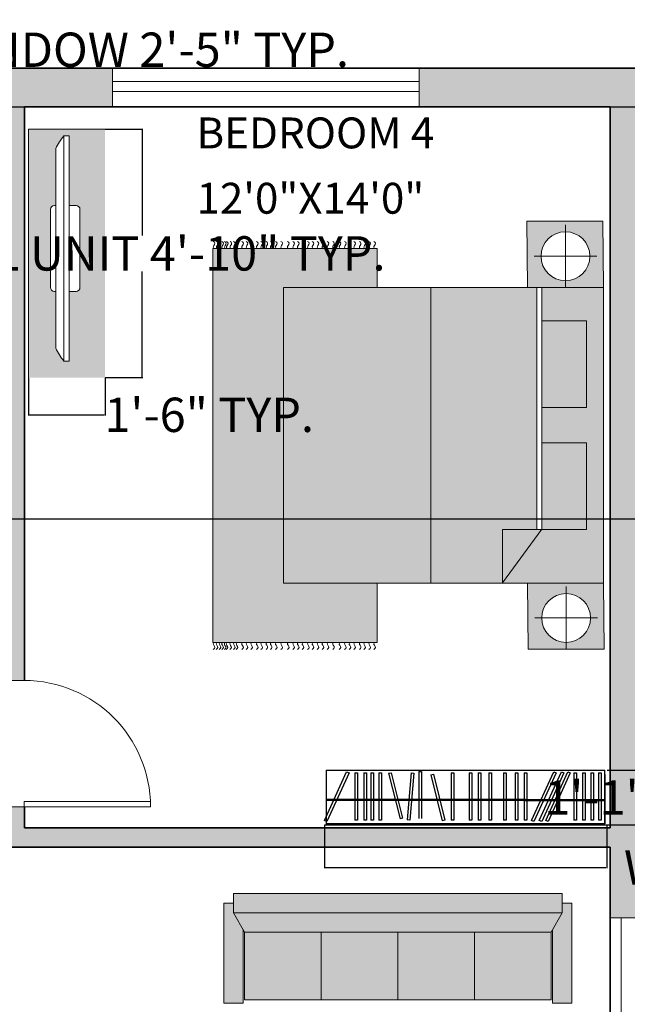
# Model space of a CAD drawing. Units: inches. Extents: x 853 to 1550, y 485 to 1596.
# Tile 16 of 18: x 1267 to 1409, y 1208 to 1437. Entities that reach past the tile are written whole.
import ezdxf

# ---------------------------------------------------------------- set-up
doc = ezdxf.new("R2010")
doc.units = ezdxf.units.IN
doc.header["$MEASUREMENT"] = 0
for name, color, linetype, lineweight in [('A-ANNO-DIMS', 2, 'Continuous', 18), ('A-AREA-IDEN', 250, 'Continuous', 18), ('A-DOOR', 4, 'Continuous', 18), ('A-WALL-PATT', 250, 'Continuous', 13), ('closet', 32, 'Continuous', 25), ('furniture', 250, 'Continuous', 18), ('walls', 250, 'Continuous', 35), ('windows', 4, 'Continuous', 18)]:
    doc.layers.add(name, color=color, linetype=linetype, lineweight=lineweight)
doc.layers.add('A-FURN-PATT', color=254, linetype='Continuous', lineweight=13, true_color=0xfeeab9)
doc.styles.get("Standard").update_dxf_attribs({"font": 'arial.ttf'})
doc.dimstyles.get("Standard").update_dxf_attribs({"dimtxt": 8, "dimasz": 0.18, "dimexe": 0.18, "dimexo": 0.0625, "dimgap": 0.09, "dimtad": 0, "dimtih": 1, "dimtoh": 1, "dimzin": 0, "dimdsep": 46, "dimlunit": 3, "dimtxsty": 'Standard', "dimcen": 0.09, "dimadec": 0, "dimazin": 0, "dimtfac": 1, "dimtofl": 0, "dimtmove": 0, "dimatfit": 3, "dimfxl": 1, "dimtolj": 1, "dimtzin": 0, "dimarcsym": 0})

# ---------------------------------------------------------------- blocks, each defined once
blk = doc.blocks.new('CARPET')
at = {"layer": 'furniture'}
for p, q in [((-51.53, -98.11), (-51.53, -55.12)), ((-51.53, -55.12), (-41.27, -55.12)), ((36, -55.12), (51.55, -55.12)), ((51.55, -55.12), (51.55, -98.11)), ((51.55, -98.11), (-51.53, -98.11))]:
    blk.add_line(p, q, dxfattribs=at)
for points, knots in [([(-53.37, -55.99), (-53.22, -55.8), (-52.9, -55.41), (-52.34, -55.8), (-51.89, -56.08), (-51.65, -55.91), (-51.53, -55.83)], [0, 0, 0, 0, 0.653278, 1.290138, 1.740457, 2.114451, 2.114451, 2.114451, 2.114451]), ([(53.37, -55.99), (53.22, -55.8), (52.9, -55.41), (52.34, -55.8), (51.89, -56.08), (51.65, -55.91), (51.53, -55.83)], [0, 0, 0, 0, 0.653278, 1.290138, 1.740457, 2.114451, 2.114451, 2.114451, 2.114451]), ([(-53.37, -57.26), (-53.22, -57.07), (-52.9, -56.67), (-52.34, -57.07), (-51.89, -57.35), (-51.65, -57.17), (-51.53, -57.1)], [0, 0, 0, 0, 0.653278, 1.290138, 1.740457, 2.114451, 2.114451, 2.114451, 2.114451]), ([(-53.37, -58.59), (-53.22, -58.4), (-52.9, -58.01), (-52.34, -58.4), (-51.89, -58.68), (-51.65, -58.5), (-51.53, -58.43)], [0, 0, 0, 0, 0.653278, 1.290138, 1.740457, 2.114451, 2.114451, 2.114451, 2.114451]), ([(53.37, -57.26), (53.22, -57.07), (52.9, -56.67), (52.34, -57.07), (51.89, -57.35), (51.65, -57.17), (51.53, -57.1)], [0, 0, 0, 0, 0.653278, 1.290138, 1.740457, 2.114451, 2.114451, 2.114451, 2.114451]), ([(53.37, -58.59), (53.22, -58.4), (52.9, -58.01), (52.34, -58.4), (51.89, -58.68), (51.65, -58.5), (51.53, -58.43)], [0, 0, 0, 0, 0.653278, 1.290138, 1.740457, 2.114451, 2.114451, 2.114451, 2.114451]), ([(-53.37, -59.78), (-53.22, -59.58), (-52.9, -59.19), (-52.34, -59.58), (-51.89, -59.86), (-51.65, -59.69), (-51.53, -59.61)], [0, 0, 0, 0, 0.653278, 1.290138, 1.740457, 2.114451, 2.114451, 2.114451, 2.114451]), ([(-53.37, -61.22), (-53.22, -61.02), (-52.9, -60.63), (-52.34, -61.02), (-51.89, -61.3), (-51.65, -61.13), (-51.53, -61.05)], [0, 0, 0, 0, 0.653278, 1.290138, 1.740457, 2.114451, 2.114451, 2.114451, 2.114451]), ([(53.37, -59.78), (53.22, -59.58), (52.9, -59.19), (52.34, -59.58), (51.89, -59.86), (51.65, -59.69), (51.53, -59.61)], [0, 0, 0, 0, 0.653278, 1.290138, 1.740457, 2.114451, 2.114451, 2.114451, 2.114451]), ([(53.37, -61.22), (53.22, -61.02), (52.9, -60.63), (52.34, -61.02), (51.89, -61.3), (51.65, -61.13), (51.53, -61.05)], [0, 0, 0, 0, 0.653278, 1.290138, 1.740457, 2.114451, 2.114451, 2.114451, 2.114451]), ([(-53.37, -62.44), (-53.22, -62.25), (-52.9, -61.86), (-52.34, -62.25), (-51.89, -62.53), (-51.65, -62.36), (-51.53, -62.28)], [0, 0, 0, 0, 0.653278, 1.290138, 1.740457, 2.114451, 2.114451, 2.114451, 2.114451]), ([(-53.37, -63.63), (-53.22, -63.43), (-52.9, -63.04), (-52.34, -63.43), (-51.89, -63.72), (-51.65, -63.54), (-51.53, -63.46)], [0, 0, 0, 0, 0.653278, 1.290138, 1.740457, 2.114451, 2.114451, 2.114451, 2.114451]), ([(53.37, -62.44), (53.22, -62.25), (52.9, -61.86), (52.34, -62.25), (51.89, -62.53), (51.65, -62.36), (51.53, -62.28)], [0, 0, 0, 0, 0.653278, 1.290138, 1.740457, 2.114451, 2.114451, 2.114451, 2.114451]), ([(53.37, -63.63), (53.22, -63.43), (52.9, -63.04), (52.34, -63.43), (51.89, -63.72), (51.65, -63.54), (51.53, -63.46)], [0, 0, 0, 0, 0.653278, 1.290138, 1.740457, 2.114451, 2.114451, 2.114451, 2.114451]), ([(-53.37, -65.07), (-53.22, -64.87), (-52.9, -64.48), (-52.34, -64.87), (-51.89, -65.15), (-51.65, -64.98), (-51.53, -64.9)], [0, 0, 0, 0, 0.653278, 1.290138, 1.740457, 2.114451, 2.114451, 2.114451, 2.114451]), ([(-53.37, -66.76), (-53.22, -66.56), (-52.9, -66.17), (-52.34, -66.56), (-51.89, -66.84), (-51.65, -66.67), (-51.53, -66.59)], [0, 0, 0, 0, 0.653278, 1.290138, 1.740457, 2.114451, 2.114451, 2.114451, 2.114451]), ([(53.37, -65.07), (53.22, -64.87), (52.9, -64.48), (52.34, -64.87), (51.89, -65.15), (51.65, -64.98), (51.53, -64.9)], [0, 0, 0, 0, 0.653278, 1.290138, 1.740457, 2.114451, 2.114451, 2.114451, 2.114451]), ([(53.37, -66.76), (53.22, -66.56), (52.9, -66.17), (52.34, -66.56), (51.89, -66.84), (51.65, -66.67), (51.53, -66.59)], [0, 0, 0, 0, 0.653278, 1.290138, 1.740457, 2.114451, 2.114451, 2.114451, 2.114451]), ([(-53.37, -68.2), (-53.22, -68), (-52.9, -67.61), (-52.34, -68), (-51.89, -68.28), (-51.65, -68.11), (-51.53, -68.03)], [0, 0, 0, 0, 0.653278, 1.290138, 1.740457, 2.114451, 2.114451, 2.114451, 2.114451]), ([(-53.37, -69.53), (-53.22, -69.33), (-52.9, -68.94), (-52.34, -69.33), (-51.89, -69.61), (-51.65, -69.44), (-51.53, -69.36)], [0, 0, 0, 0, 0.653278, 1.290138, 1.740457, 2.114451, 2.114451, 2.114451, 2.114451]), ([(53.37, -68.2), (53.22, -68), (52.9, -67.61), (52.34, -68), (51.89, -68.28), (51.65, -68.11), (51.53, -68.03)], [0, 0, 0, 0, 0.653278, 1.290138, 1.740457, 2.114451, 2.114451, 2.114451, 2.114451]), ([(53.37, -69.53), (53.22, -69.33), (52.9, -68.94), (52.34, -69.33), (51.89, -69.61), (51.65, -69.44), (51.53, -69.36)], [0, 0, 0, 0, 0.653278, 1.290138, 1.740457, 2.114451, 2.114451, 2.114451, 2.114451]), ([(-53.37, -70.79), (-53.22, -70.6), (-52.9, -70.21), (-52.34, -70.6), (-51.89, -70.88), (-51.65, -70.7), (-51.53, -70.63)], [0, 0, 0, 0, 0.653278, 1.290138, 1.740457, 2.114451, 2.114451, 2.114451, 2.114451]), ([(-53.37, -72.12), (-53.22, -71.93), (-52.9, -71.54), (-52.34, -71.93), (-51.89, -72.21), (-51.65, -72.04), (-51.53, -71.96)], [0, 0, 0, 0, 0.653278, 1.290138, 1.740457, 2.114451, 2.114451, 2.114451, 2.114451]), ([(53.37, -70.79), (53.22, -70.6), (52.9, -70.21), (52.34, -70.6), (51.89, -70.88), (51.65, -70.7), (51.53, -70.63)], [0, 0, 0, 0, 0.653278, 1.290138, 1.740457, 2.114451, 2.114451, 2.114451, 2.114451]), ([(53.37, -72.12), (53.22, -71.93), (52.9, -71.54), (52.34, -71.93), (51.89, -72.21), (51.65, -72.04), (51.53, -71.96)], [0, 0, 0, 0, 0.653278, 1.290138, 1.740457, 2.114451, 2.114451, 2.114451, 2.114451]), ([(-53.37, -73.31), (-53.22, -73.11), (-52.9, -72.72), (-52.34, -73.11), (-51.89, -73.4), (-51.65, -73.22), (-51.53, -73.14)], [0, 0, 0, 0, 0.653278, 1.290138, 1.740457, 2.114451, 2.114451, 2.114451, 2.114451]), ([(-53.37, -74.75), (-53.22, -74.55), (-52.9, -74.16), (-52.34, -74.55), (-51.89, -74.83), (-51.65, -74.66), (-51.53, -74.58)], [0, 0, 0, 0, 0.653278, 1.290138, 1.740457, 2.114451, 2.114451, 2.114451, 2.114451]), ([(53.37, -73.31), (53.22, -73.11), (52.9, -72.72), (52.34, -73.11), (51.89, -73.4), (51.65, -73.22), (51.53, -73.14)], [0, 0, 0, 0, 0.653278, 1.290138, 1.740457, 2.114451, 2.114451, 2.114451, 2.114451]), ([(53.37, -74.75), (53.22, -74.55), (52.9, -74.16), (52.34, -74.55), (51.89, -74.83), (51.65, -74.66), (51.53, -74.58)], [0, 0, 0, 0, 0.653278, 1.290138, 1.740457, 2.114451, 2.114451, 2.114451, 2.114451]), ([(-53.37, -75.98), (-53.22, -75.78), (-52.9, -75.39), (-52.34, -75.78), (-51.89, -76.06), (-51.65, -75.89), (-51.53, -75.81)], [0, 0, 0, 0, 0.653278, 1.290138, 1.740457, 2.114451, 2.114451, 2.114451, 2.114451]), ([(-53.37, -77.16), (-53.22, -76.96), (-52.9, -76.57), (-52.34, -76.96), (-51.89, -77.25), (-51.65, -77.07), (-51.53, -76.99)], [0, 0, 0, 0, 0.653278, 1.290138, 1.740457, 2.114451, 2.114451, 2.114451, 2.114451]), ([(53.37, -75.98), (53.22, -75.78), (52.9, -75.39), (52.34, -75.78), (51.89, -76.06), (51.65, -75.89), (51.53, -75.81)], [0, 0, 0, 0, 0.653278, 1.290138, 1.740457, 2.114451, 2.114451, 2.114451, 2.114451]), ([(53.37, -77.16), (53.22, -76.96), (52.9, -76.57), (52.34, -76.96), (51.89, -77.25), (51.65, -77.07), (51.53, -76.99)], [0, 0, 0, 0, 0.653278, 1.290138, 1.740457, 2.114451, 2.114451, 2.114451, 2.114451]), ([(-53.37, -78.6), (-53.22, -78.4), (-52.9, -78.01), (-52.34, -78.4), (-51.89, -78.68), (-51.65, -78.51), (-51.53, -78.43)], [0, 0, 0, 0, 0.653278, 1.290138, 1.740457, 2.114451, 2.114451, 2.114451, 2.114451]), ([(53.37, -78.6), (53.22, -78.4), (52.9, -78.01), (52.34, -78.4), (51.89, -78.68), (51.65, -78.51), (51.53, -78.43)], [0, 0, 0, 0, 0.653278, 1.290138, 1.740457, 2.114451, 2.114451, 2.114451, 2.114451]), ([(-53.37, -80.29), (-53.22, -80.09), (-52.9, -79.7), (-52.34, -80.09), (-51.89, -80.37), (-51.65, -80.2), (-51.53, -80.12)], [0, 0, 0, 0, 0.653278, 1.290138, 1.740457, 2.114451, 2.114451, 2.114451, 2.114451]), ([(-53.37, -81.73), (-53.22, -81.53), (-52.9, -81.14), (-52.34, -81.53), (-51.89, -81.81), (-51.65, -81.64), (-51.53, -81.56)], [0, 0, 0, 0, 0.653278, 1.290138, 1.740457, 2.114451, 2.114451, 2.114451, 2.114451]), ([(53.37, -80.29), (53.22, -80.09), (52.9, -79.7), (52.34, -80.09), (51.89, -80.37), (51.65, -80.2), (51.53, -80.12)], [0, 0, 0, 0, 0.653278, 1.290138, 1.740457, 2.114451, 2.114451, 2.114451, 2.114451]), ([(53.37, -81.73), (53.22, -81.53), (52.9, -81.14), (52.34, -81.53), (51.89, -81.81), (51.65, -81.64), (51.53, -81.56)], [0, 0, 0, 0, 0.653278, 1.290138, 1.740457, 2.114451, 2.114451, 2.114451, 2.114451]), ([(-53.37, -83.06), (-53.22, -82.86), (-52.9, -82.47), (-52.34, -82.86), (-51.89, -83.14), (-51.65, -82.97), (-51.53, -82.89)], [0, 0, 0, 0, 0.653278, 1.290138, 1.740457, 2.114451, 2.114451, 2.114451, 2.114451]), ([(-53.37, -84.18), (-53.22, -83.99), (-52.9, -83.6), (-52.34, -83.99), (-51.89, -84.27), (-51.65, -84.09), (-51.53, -84.02)], [0, 0, 0, 0, 0.653278, 1.290138, 1.740457, 2.114451, 2.114451, 2.114451, 2.114451]), ([(53.37, -83.06), (53.22, -82.86), (52.9, -82.47), (52.34, -82.86), (51.89, -83.14), (51.65, -82.97), (51.53, -82.89)], [0, 0, 0, 0, 0.653278, 1.290138, 1.740457, 2.114451, 2.114451, 2.114451, 2.114451]), ([(53.37, -84.18), (53.22, -83.99), (52.9, -83.6), (52.34, -83.99), (51.89, -84.27), (51.65, -84.09), (51.53, -84.02)], [0, 0, 0, 0, 0.653278, 1.290138, 1.740457, 2.114451, 2.114451, 2.114451, 2.114451]), ([(-53.37, -85.51), (-53.22, -85.32), (-52.9, -84.93), (-52.34, -85.32), (-51.89, -85.6), (-51.65, -85.42), (-51.53, -85.35)], [0, 0, 0, 0, 0.653278, 1.290138, 1.740457, 2.114451, 2.114451, 2.114451, 2.114451]), ([(-53.37, -86.7), (-53.22, -86.5), (-52.9, -86.11), (-52.34, -86.5), (-51.89, -86.78), (-51.65, -86.61), (-51.53, -86.53)], [0, 0, 0, 0, 0.653278, 1.290138, 1.740457, 2.114451, 2.114451, 2.114451, 2.114451]), ([(53.37, -85.51), (53.22, -85.32), (52.9, -84.93), (52.34, -85.32), (51.89, -85.6), (51.65, -85.42), (51.53, -85.35)], [0, 0, 0, 0, 0.653278, 1.290138, 1.740457, 2.114451, 2.114451, 2.114451, 2.114451]), ([(53.37, -86.7), (53.22, -86.5), (52.9, -86.11), (52.34, -86.5), (51.89, -86.78), (51.65, -86.61), (51.53, -86.53)], [0, 0, 0, 0, 0.653278, 1.290138, 1.740457, 2.114451, 2.114451, 2.114451, 2.114451]), ([(-53.37, -88.14), (-53.22, -87.94), (-52.9, -87.55), (-52.34, -87.94), (-51.89, -88.22), (-51.65, -88.05), (-51.53, -87.97)], [0, 0, 0, 0, 0.653278, 1.290138, 1.740457, 2.114451, 2.114451, 2.114451, 2.114451]), ([(-53.37, -89.36), (-53.22, -89.17), (-52.9, -88.78), (-52.34, -89.17), (-51.89, -89.45), (-51.65, -89.28), (-51.53, -89.2)], [0, 0, 0, 0, 0.653278, 1.290138, 1.740457, 2.114451, 2.114451, 2.114451, 2.114451]), ([(-53.37, -90.55), (-53.22, -90.35), (-52.9, -89.96), (-52.34, -90.35), (-51.89, -90.64), (-51.65, -90.46), (-51.53, -90.38)], [0, 0, 0, 0, 0.653278, 1.290138, 1.740457, 2.114451, 2.114451, 2.114451, 2.114451]), ([(53.37, -88.14), (53.22, -87.94), (52.9, -87.55), (52.34, -87.94), (51.89, -88.22), (51.65, -88.05), (51.53, -87.97)], [0, 0, 0, 0, 0.653278, 1.290138, 1.740457, 2.114451, 2.114451, 2.114451, 2.114451]), ([(53.37, -89.36), (53.22, -89.17), (52.9, -88.78), (52.34, -89.17), (51.89, -89.45), (51.65, -89.28), (51.53, -89.2)], [0, 0, 0, 0, 0.653278, 1.290138, 1.740457, 2.114451, 2.114451, 2.114451, 2.114451]), ([(53.37, -90.55), (53.22, -90.35), (52.9, -89.96), (52.34, -90.35), (51.9, -90.63), (51.66, -90.47), (51.55, -90.4)], [0, 0, 0, 0, 0.653278, 1.290138, 1.740457, 2.0926, 2.0926, 2.0926, 2.0926]), ([(-53.37, -91.99), (-53.22, -91.79), (-52.9, -91.4), (-52.34, -91.79), (-51.89, -92.07), (-51.65, -91.9), (-51.53, -91.82)], [0, 0, 0, 0, 0.653278, 1.290138, 1.740457, 2.114451, 2.114451, 2.114451, 2.114451]), ([(-53.37, -92.69), (-53.22, -92.48), (-52.9, -92.08), (-52.35, -92.49), (-51.89, -92.77), (-51.65, -92.6), (-51.53, -92.52)], [0, 0, 0, 0, 0.663904, 1.307406, 1.757725, 2.131719, 2.131719, 2.131719, 2.131719]), ([(53.37, -91.99), (53.22, -91.79), (52.9, -91.4), (52.34, -91.79), (51.9, -92.07), (51.66, -91.91), (51.55, -91.83)], [0, 0, 0, 0, 0.653278, 1.290138, 1.740457, 2.0926, 2.0926, 2.0926, 2.0926]), ([(53.37, -92.69), (53.22, -92.49), (52.9, -92.09), (52.34, -92.49), (51.9, -92.77), (51.66, -92.61), (51.55, -92.53)], [0, 0, 0, 0, 0.656792, 1.295826, 1.746145, 2.098292, 2.098292, 2.098292, 2.098292]), ([(-53.37, -93.61), (-53.22, -93.42), (-52.9, -93.03), (-52.34, -93.42), (-51.89, -93.7), (-51.65, -93.52), (-51.53, -93.45)], [0, 0, 0, 0, 0.653278, 1.290138, 1.740457, 2.114451, 2.114451, 2.114451, 2.114451]), ([(-53.37, -94.55), (-53.22, -94.35), (-52.9, -93.96), (-52.34, -94.35), (-51.89, -94.63), (-51.65, -94.46), (-51.53, -94.38)], [0, 0, 0, 0, 0.653278, 1.290138, 1.740457, 2.114451, 2.114451, 2.114451, 2.114451]), ([(-53.37, -95.05), (-53.22, -94.85), (-52.9, -94.46), (-52.34, -94.85), (-51.89, -95.14), (-51.65, -94.96), (-51.53, -94.88)], [0, 0, 0, 0, 0.653278, 1.290138, 1.740457, 2.114451, 2.114451, 2.114451, 2.114451]), ([(53.37, -93.66), (53.22, -93.46), (52.9, -93.07), (52.34, -93.46), (51.9, -93.74), (51.66, -93.58), (51.55, -93.5)], [0, 0, 0, 0, 0.653278, 1.290138, 1.740457, 2.0926, 2.0926, 2.0926, 2.0926]), ([(53.37, -94.59), (53.22, -94.4), (52.9, -94.01), (52.34, -94.4), (51.9, -94.68), (51.66, -94.51), (51.55, -94.44)], [0, 0, 0, 0, 0.653278, 1.290138, 1.740457, 2.0926, 2.0926, 2.0926, 2.0926]), ([(53.37, -95.1), (53.22, -94.9), (52.9, -94.51), (52.34, -94.9), (51.9, -95.18), (51.66, -95.02), (51.55, -94.94)], [0, 0, 0, 0, 0.653278, 1.290138, 1.740457, 2.0926, 2.0926, 2.0926, 2.0926]), ([(-53.37, -95.73), (-53.22, -95.54), (-52.9, -95.15), (-52.34, -95.54), (-51.89, -95.82), (-51.65, -95.65), (-51.53, -95.57)], [0, 0, 0, 0, 0.653278, 1.290138, 1.740457, 2.114451, 2.114451, 2.114451, 2.114451]), ([(-53.37, -96.38), (-53.22, -96.18), (-52.9, -95.79), (-52.34, -96.18), (-51.89, -96.47), (-51.65, -96.29), (-51.53, -96.21)], [0, 0, 0, 0, 0.653278, 1.290138, 1.740457, 2.114451, 2.114451, 2.114451, 2.114451]), ([(-53.37, -97.17), (-53.22, -96.98), (-52.9, -96.59), (-52.34, -96.98), (-51.89, -97.26), (-51.65, -97.08), (-51.53, -97.01)], [0, 0, 0, 0, 0.653278, 1.290138, 1.740457, 2.114451, 2.114451, 2.114451, 2.114451]), ([(-53.37, -97.99), (-53.22, -97.79), (-52.9, -97.4), (-52.34, -97.79), (-51.89, -98.08), (-51.65, -97.9), (-51.53, -97.82)], [0, 0, 0, 0, 0.653278, 1.290138, 1.740457, 2.114451, 2.114451, 2.114451, 2.114451]), ([(53.37, -95.78), (53.22, -95.58), (52.9, -95.19), (52.34, -95.58), (51.89, -95.86), (51.65, -95.69), (51.53, -95.61)], [0, 0, 0, 0, 0.653278, 1.290138, 1.740457, 2.114451, 2.114451, 2.114451, 2.114451]), ([(53.37, -96.43), (53.22, -96.23), (52.9, -95.84), (52.34, -96.23), (51.89, -96.51), (51.65, -96.34), (51.53, -96.26)], [0, 0, 0, 0, 0.653278, 1.290138, 1.740457, 2.114451, 2.114451, 2.114451, 2.114451]), ([(53.37, -97.22), (53.22, -97.02), (52.9, -96.63), (52.34, -97.02), (51.89, -97.3), (51.65, -97.13), (51.53, -97.05)], [0, 0, 0, 0, 0.653278, 1.290138, 1.740457, 2.114451, 2.114451, 2.114451, 2.114451]), ([(53.37, -97.99), (53.22, -97.79), (52.9, -97.4), (52.34, -97.79), (51.89, -98.08), (51.65, -97.9), (51.53, -97.82)], [0, 0, 0, 0, 0.653278, 1.290138, 1.740457, 2.114451, 2.114451, 2.114451, 2.114451])]:
    blk.add_open_spline(points, degree=3, knots=knots, dxfattribs=at)
blk = doc.blocks.new('A$C58D270C6')
at = {"layer": 'furniture'}
for p, q in [((9.09, 124.13), (9.09, 108.87)), ((1.46, 116.5), (16.73, 116.5)), ((42.08, 108), (42.08, 36)), ((14.97, 94.84), (24.62, 107.92)), ((24.62, 94.93), (24.62, 107.92)), ((14.97, 94.93), (24.62, 94.93)), ((14.97, 94.84), (14.97, 36)), ((16.22, 94.93), (16.22, 36)), ((9.25, 36), (9.25, 20.74)), ((1.62, 28.37), (16.88, 28.37))]:
    blk.add_line(p, q, dxfattribs=at)
for points in [[(18.5, 108), (18.34, 124.13), (-0.16, 124.13), (0, 108)], [(0, 108), (77.91, 108), (77.91, 36), (0, 36)], [(4.09, 94.93), (14.97, 94.93), (14.97, 73.83), (4.09, 73.83)], [(4.09, 65.23), (14.97, 65.23), (14.97, 44.13), (4.09, 44.13)], [(18.65, 19.87), (18.5, 36), (0, 36), (0.16, 19.87)]]:
    blk.add_lwpolyline(points, close=True, dxfattribs=at)
for centre in [(9.09, 116.5), (9.25, 28.37)]:
    blk.add_circle(centre, 5.95, dxfattribs=at)
at = {"layer": 'furniture', "xscale": 0.9312884925094044, "yscale": 0.9312884925094044, "zscale": 0.9312884925094044, "rotation": 90}
blk.add_blockref('CARPET', (3.79, 74.47), dxfattribs=at)
blk = doc.blocks.new('*U10')
for p, q in [((0, 0), (0, -6)), ((40, 0), (40, -6))]:
    blk.add_line(p, q)
blk.add_lwpolyline([(0, 0), (0, 40), (1.75, 40), (1.75, 0)], close=True)
blk.add_arc((0, 0), 40, 0, 90)
blk = doc.blocks.new('FABRIC SOFA 4S')
at = {"layer": 'furniture'}
for p, q in [((3, 54), (34, 54)), ((3, 51), (3, 54)), ((34, 48), (34, 54)), ((0, -51), (0, 51)), ((6, 51), (0, 51)), ((6, -51), (6, 51)), ((12, 47.63), (6, 51)), ((11.14, 48), (34, 48)), ((33, 23.81), (12, 23.81)), ((33, 0), (12, 0)), ((33, -23.81), (12, -23.81)), ((6, -51), (12, -47.63)), ((11.54, -48), (34, -48)), ((34, -48), (34, -54)), ((6, -51), (0, -51)), ((3, -54), (3, -51)), ((3, -54), (34, -54))]:
    blk.add_line(p, q, dxfattribs=at)
blk.add_lwpolyline([(12, -47.63), (12, 47.63), (33, 47.63), (33, -47.63)], close=True, dxfattribs=at)
blk = doc.blocks.new('WIN-71IN')
for p, q in [((0, 9), (0, 0)), ((71.43, 9), (0, 9)), ((0, 9), (0, 5.92)), ((71.43, 0), (71.43, 9)), ((0, 5.92), (71.43, 5.92)), ((71.43, 5.92), (71.43, 3.59)), ((71.43, 3.59), (0, 3.59)), ((0, 0), (71.43, 0))]:
    blk.add_line(p, q)
blk = doc.blocks.new('WIN-94IN')
for p, q in [((0, 94.25), (9, 94.25)), ((0, 0), (0, 94.25)), ((2.54, 94.25), (2.54, 0)), ((6.1, 0), (6.1, 94.25)), ((9, 94.25), (9, 0)), ((9, 0), (0, 0)), ((2.54, 0), (6.1, 0))]:
    blk.add_line(p, q)
blk = doc.blocks.new('closet')
at = {"layer": 'closet'}
for p, q in [((-0.71, -5.58), (5.59, 8.19)), ((-0.23, 7.39), (-0.23, -6.57)), ((6.27, 7.88), (-0.04, -5.89)), ((5.59, 8.19), (6.27, 7.88)), ((7.92, 7.84), (8.68, 7.84)), ((7.92, 7.84), (7.92, -5.51)), ((8.68, 7.84), (8.68, -5.51)), ((10.44, 7.84), (11.2, 7.84)), ((10.44, 7.84), (10.44, -5.51)), ((11.2, 7.84), (11.2, -5.51)), ((12.45, 7.84), (13.21, 7.84)), ((12.45, 7.84), (12.45, -5.51)), ((13.21, 7.84), (13.21, -5.51)), ((14.71, 7.84), (15.47, 7.84)), ((14.71, 7.84), (14.71, -5.51)), ((15.47, 7.84), (15.47, -5.51)), ((17.44, 7.75), (18.17, 7.93)), ((17.44, 7.75), (20.73, -5.2)), ((18.17, 7.93), (21.46, -5.01)), ((23.92, 7.84), (22.75, -5.46)), ((24.67, 7.78), (23.51, -5.53)), ((23.92, 7.84), (24.67, 7.78)), ((26.09, 8.25), (26.09, -5.1)), ((26.84, 8.25), (26.84, -5.1)), ((29.49, 7.29), (32.64, -5.69)), ((30.22, 7.46), (33.37, -5.51)), ((35.23, 7.84), (35.23, -5.51)), ((35.99, 7.84), (35.99, -5.51)), ((40.33, 7.84), (40.33, -5.51)), ((41.08, 7.84), (41.08, -5.51)), ((42.85, 7.84), (42.85, -5.51)), ((43.61, 7.84), (43.61, -5.51)), ((45.9, 7.84), (45.9, -5.51)), ((46.65, 7.84), (46.65, -5.51)), ((50.07, 7.84), (50.07, -5.51)), ((50.82, 7.84), (50.82, -5.51)), ((53.32, 7.84), (53.32, -5.51)), ((54.08, 7.84), (54.08, -5.51)), ((55.9, 7.84), (55.9, -5.51)), ((56.65, 7.84), (56.65, -5.51)), ((57.99, -5.58), (64.3, 8.19)), ((64.97, 7.88), (58.67, -5.89)), ((60.19, -5.58), (66.49, 8.19)), ((67.17, 7.88), (60.87, -5.89)), ((62, -5.58), (68.3, 8.19)), ((68.98, 7.88), (62.67, -5.89)), ((69.96, 7.84), (69.96, -5.51)), ((70.72, 7.84), (70.72, -5.51)), ((72.43, 7.84), (72.43, -5.51)), ((73.19, 7.84), (73.19, -5.51)), ((74.82, 7.84), (74.82, -5.51)), ((75.57, 7.84), (75.57, -5.51)), ((76.94, 7.84), (76.94, -5.51)), ((77.69, 7.84), (77.69, -5.51)), ((56.23, 0.33), (0, 0.33)), ((56.2, 0), (0, 0)), ((56.2, 0), (78.76, 0)), ((56.23, 0.33), (78.76, 0.33)), ((-0.04, -5.89), (-0.71, -5.58)), ((21.46, -5.01), (20.73, -5.2)), ((23.51, -5.53), (22.75, -5.46)), ((33.37, -5.51), (32.64, -5.69)), ((35.99, -5.51), (35.23, -5.51)), ((41.08, -5.51), (40.33, -5.51)), ((43.61, -5.51), (42.85, -5.51)), ((46.65, -5.51), (45.9, -5.51)), ((50.82, -5.51), (50.07, -5.51)), ((54.08, -5.51), (53.32, -5.51)), ((56.65, -5.51), (55.9, -5.51)), ((58.67, -5.89), (57.99, -5.58)), ((60.87, -5.89), (60.19, -5.58)), ((62.67, -5.89), (62, -5.58)), ((70.72, -5.51), (69.96, -5.51)), ((73.19, -5.51), (72.43, -5.51)), ((75.57, -5.51), (74.82, -5.51)), ((77.69, -5.51), (76.94, -5.51))]:
    blk.add_line(p, q, dxfattribs=at)
blk = doc.blocks.new('rotated closet')
at = {"layer": 'closet'}
for p, q in [((26.32, 0.86), (27.07, 0.86)), ((29.72, -0.11), (30.45, 0.07)), ((35.46, 0.45), (36.22, 0.45)), ((40.56, 0.45), (41.31, 0.45)), ((43.08, 0.45), (43.84, 0.45)), ((46.13, 0.45), (46.88, 0.45)), ((50.3, 0.45), (51.05, 0.45)), ((53.56, 0.45), (54.31, 0.45)), ((56.13, 0.45), (56.88, 0.45)), ((64.53, 0.8), (65.2, 0.49)), ((66.72, 0.8), (67.4, 0.49)), ((68.53, 0.8), (69.21, 0.49)), ((70.19, 0.45), (70.95, 0.45)), ((72.66, 0.45), (73.42, 0.45)), ((75.05, 0.45), (75.81, 0.45)), ((77.17, 0.45), (77.92, 0.45)), ((78.99, 0), (78.99, -13.96)), ((8.91, -12.91), (8.15, -12.91)), ((11.43, -12.91), (10.67, -12.91)), ((13.44, -12.91), (12.68, -12.91)), ((15.7, -12.91), (14.94, -12.91)), ((-0.46, -14.27), (79.54, -14.27)), ((0, -13.96), (78.99, -13.96))]:
    blk.add_line(p, q, dxfattribs=at)
blk.add_blockref('closet', (0.23, -7.39), dxfattribs=at)
blk = doc.blocks.new('WARDROBE-FRAMED')
for p, q in [((0.4, 12.8), (65.33, 12.8)), ((0.4, 12.8), (0.4, 0.26)), ((65.33, 0.26), (65.33, 12.8)), ((0.02, 0), (65.79, 0)), ((65.33, 0.26), (0.4, 0.26)), ((0.4, 0.26), (0.4, 0))]:
    blk.add_line(p, q)
at = {"xscale": 0.8221057635095903, "yscale": 0.8221057635095903, "zscale": 0.8221057635095903, "rotation": 359.9999999992008}
blk.add_blockref('rotated closet', (0.4, 11.74), dxfattribs=at)
blk = doc.blocks.new('PLASMA-LARGE')
at = {"layer": 'furniture'}
for p, q in [((-7.26, 0), (7.26, 0)), ((-18.61, -1), (18.61, -1)), ((-8, -1), (-8, -0.74)), ((8, -1), (8, -0.74)), ((-21, -2.5), (21, -2.5)), ((-21, -2.5), (-21, -3.5)), ((-21, -3.5), (21, -3.5)), ((-8, -3.5), (-8, -4.76)), ((8, -3.5), (8, -4.76)), ((21, -2.5), (21, -3.5)), ((-7.26, -5.5), (7.26, -5.5))]:
    blk.add_line(p, q, dxfattribs=at)
for centre, radius, start, end in [((-7.26, -0.74), 0.744, 90, 180), ((7.26, -0.74), 0.744, 0, 90), ((-13.97, -11.05), 11.07, 114.7602, 129.4175), ((13.97, -11.05), 11.07, 50.5825, 65.2398), ((-7.26, -4.76), 0.744, 180, 270), ((7.26, -4.76), 0.744, 270, 0)]:
    blk.add_arc(centre, radius, start, end, dxfattribs=at)
blk = doc.blocks.new('TV-CONSOLE-WALL')
for p, q in [((17.81, 57.83), (0, 57.83)), ((0, 57.83), (0, 0))]:
    blk.add_line(p, q)
at = {"xscale": -1.249763490704796, "yscale": 1.249763490704796, "zscale": 1.249763490704796, "rotation": 90}
blk.add_blockref('PLASMA-LARGE', (5.11, 30.08), dxfattribs=at)
blk = doc.blocks.new('*D43')
at = {"layer": 'A-ANNO-DIMS', "color": 0, "lineweight": -2, "transparency": 16777216}
for p, q in [((1338.32, 1249.77), (1338.32, 1239.78)), ((1404.11, 1249.77), (1404.11, 1239.78)), ((1338.5, 1239.96), (1403.93, 1239.96)), ((1404.11, 1239.96), (1404.29, 1239.96))]:
    blk.add_line(p, q, dxfattribs=at)
at = {"layer": 'A-ANNO-DIMS', "color": 0, "transparency": 16777216}
for points in [[(1338.5, 1239.99), (1338.5, 1239.93), (1338.32, 1239.96)], [(1403.93, 1239.99), (1403.93, 1239.93), (1404.11, 1239.96)]]:
    blk.add_solid(points, dxfattribs=at)
at = {"layer": 'Defpoints', "color": 0, "transparency": 16777216}
for p in [(1338.32, 1249.83), (1404.11, 1249.83), (1404.11, 1239.96)]:
    blk.add_point(p, dxfattribs=at)
at = {"layer": 'A-ANNO-DIMS', "color": 0, "transparency": 16777216, "insert": (1463.39, 1239.96), "char_height": 8, "attachment_point": 5}
blk.add_mtext('\\A1;WARDROBE 5\'-6" TYP.', dxfattribs=at)
blk = doc.blocks.new('*D44')
at = {"layer": 'A-ANNO-DIMS', "color": 0, "lineweight": -2, "transparency": 16777216}
for p, q in [((1404.17, 1262.63), (1414.16, 1262.63)), ((1413.98, 1262.45), (1413.98, 1260.34)), ((1413.98, 1250.01), (1413.98, 1252.12)), ((1404.17, 1249.83), (1414.16, 1249.83))]:
    blk.add_line(p, q, dxfattribs=at)
at = {"layer": 'A-ANNO-DIMS', "color": 0, "transparency": 16777216}
for points in [[(1413.95, 1262.45), (1414.01, 1262.45), (1413.98, 1262.63)], [(1413.95, 1250.01), (1414.01, 1250.01), (1413.98, 1249.83)]]:
    blk.add_solid(points, dxfattribs=at)
at = {"layer": 'Defpoints', "color": 0, "transparency": 16777216}
for p in [(1404.11, 1262.63), (1413.98, 1262.63), (1404.11, 1249.83)]:
    blk.add_point(p, dxfattribs=at)
at = {"layer": 'A-ANNO-DIMS', "color": 0, "transparency": 16777216, "insert": (1413.98, 1256.23), "char_height": 8, "attachment_point": 5}
blk.add_mtext('\\A1;1\'-1" TYP.', dxfattribs=at)
blk = doc.blocks.new('*D51')
at = {"layer": 'A-ANNO-DIMS', "color": 0, "lineweight": -2, "transparency": 16777216}
for p, q in [((1215.84, 1426.19), (1215.84, 1430.62)), ((1216.02, 1430.44), (1244.42, 1430.44)), ((1244.6, 1426.19), (1244.6, 1430.62)), ((1244.6, 1430.44), (1244.78, 1430.44))]:
    blk.add_line(p, q, dxfattribs=at)
at = {"layer": 'A-ANNO-DIMS', "color": 0, "transparency": 16777216}
for points in [[(1216.02, 1430.47), (1216.02, 1430.41), (1215.84, 1430.44)], [(1244.42, 1430.47), (1244.42, 1430.41), (1244.6, 1430.44)]]:
    blk.add_solid(points, dxfattribs=at)
at = {"layer": 'Defpoints', "color": 0, "transparency": 16777216}
for p in [(1244.6, 1430.44), (1215.84, 1426.13), (1244.6, 1426.13)]:
    blk.add_point(p, dxfattribs=at)
at = {"layer": 'A-ANNO-DIMS', "color": 0, "transparency": 16777216, "insert": (1295.48, 1430.44), "char_height": 8, "attachment_point": 5}
blk.add_mtext('\\A1;WINDOW 2\'-5" TYP.', dxfattribs=at)
blk = doc.blocks.new('*D57')
at = {"layer": 'A-ANNO-DIMS', "color": 0, "lineweight": -2, "transparency": 16777216}
for p, q in [((1287.27, 1411.9), (1296.06, 1411.9)), ((1295.88, 1411.72), (1295.88, 1387.16)), ((1295.88, 1354.25), (1295.88, 1378.81)), ((1287.27, 1354.07), (1296.06, 1354.07))]:
    blk.add_line(p, q, dxfattribs=at)
at = {"layer": 'A-ANNO-DIMS', "color": 0, "transparency": 16777216}
for points in [[(1295.85, 1411.72), (1295.91, 1411.72), (1295.88, 1411.9)], [(1295.85, 1354.25), (1295.91, 1354.25), (1295.88, 1354.07)]]:
    blk.add_solid(points, dxfattribs=at)
at = {"layer": 'Defpoints', "color": 0, "transparency": 16777216}
for p in [(1287.21, 1411.9), (1295.88, 1411.9), (1287.21, 1354.07)]:
    blk.add_point(p, dxfattribs=at)
at = {"layer": 'A-ANNO-DIMS', "color": 0, "transparency": 16777216, "insert": (1295.88, 1382.99), "char_height": 8, "attachment_point": 5}
blk.add_mtext('\\A1;WALL UNIT 4\'-10" TYP.', dxfattribs=at)
blk = doc.blocks.new('*D58')
at = {"layer": 'A-ANNO-DIMS', "color": 0, "lineweight": -2, "transparency": 16777216}
for p, q in [((1269.39, 1354.01), (1269.39, 1345.21)), ((1287.21, 1354.01), (1287.21, 1345.21)), ((1269.57, 1345.39), (1287.03, 1345.39)), ((1287.21, 1345.39), (1287.39, 1345.39))]:
    blk.add_line(p, q, dxfattribs=at)
at = {"layer": 'A-ANNO-DIMS', "color": 0, "transparency": 16777216}
for points in [[(1269.57, 1345.42), (1269.57, 1345.36), (1269.39, 1345.39)], [(1287.03, 1345.42), (1287.03, 1345.36), (1287.21, 1345.39)]]:
    blk.add_solid(points, dxfattribs=at)
at = {"layer": 'Defpoints', "color": 0, "transparency": 16777216}
for p in [(1269.39, 1354.07), (1287.21, 1354.07), (1287.21, 1345.39)]:
    blk.add_point(p, dxfattribs=at)
at = {"layer": 'A-ANNO-DIMS', "color": 0, "transparency": 16777216, "insert": (1311.48, 1345.39), "char_height": 8, "attachment_point": 5}
blk.add_mtext('\\A1;1\'-6" TYP.', dxfattribs=at)
blk = doc.blocks.new('*D69')
at = {"layer": 'A-ANNO-DIMS', "color": 0, "lineweight": -2, "transparency": 16777216}
for p, q in [((981.94, 1426.19), (981.94, 1584.65)), ((982.12, 1584.47), (1184.11, 1584.47)), ((1413.76, 1584.47), (1211.77, 1584.47)), ((1413.94, 1426.19), (1413.94, 1584.65))]:
    blk.add_line(p, q, dxfattribs=at)
at = {"layer": 'A-ANNO-DIMS', "color": 0, "transparency": 16777216}
for points in [[(982.12, 1584.5), (982.12, 1584.44), (981.94, 1584.47)], [(1413.76, 1584.5), (1413.76, 1584.44), (1413.94, 1584.47)]]:
    blk.add_solid(points, dxfattribs=at)
at = {"layer": 'Defpoints', "color": 0, "transparency": 16777216}
for p in [(1413.94, 1584.47), (981.94, 1426.13), (1413.94, 1426.13)]:
    blk.add_point(p, dxfattribs=at)
at = {"layer": 'A-ANNO-DIMS', "color": 0, "transparency": 16777216, "insert": (1197.94, 1584.47), "char_height": 8, "attachment_point": 5}
blk.add_mtext('\\A1;36\'-0"', dxfattribs=at)
blk = doc.blocks.new('*D73')
at = {"layer": 'A-ANNO-DIMS', "color": 0, "lineweight": -2, "transparency": 16777216}
for p, q in [((1139.5, 1417.13), (1526.24, 1417.13)), ((1526.06, 1416.95), (1526.06, 1373.3)), ((1526.06, 1321.31), (1526.06, 1364.95)), ((1139.5, 1321.13), (1526.24, 1321.13))]:
    blk.add_line(p, q, dxfattribs=at)
at = {"layer": 'A-ANNO-DIMS', "color": 0, "transparency": 16777216}
for points in [[(1526.03, 1416.95), (1526.09, 1416.95), (1526.06, 1417.13)], [(1526.03, 1321.31), (1526.09, 1321.31), (1526.06, 1321.13)]]:
    blk.add_solid(points, dxfattribs=at)
at = {"layer": 'Defpoints', "color": 0, "transparency": 16777216}
for p in [(1139.44, 1417.13), (1139.44, 1321.13), (1526.06, 1321.13)]:
    blk.add_point(p, dxfattribs=at)
at = {"layer": 'A-ANNO-DIMS', "color": 0, "transparency": 16777216, "insert": (1526.06, 1369.13), "char_height": 8, "attachment_point": 5}
blk.add_mtext('\\A1;8\'-0"', dxfattribs=at)

msp = doc.modelspace()

# ---------------------------------------------------------------- hatches: boundary and pattern name
at = {"layer": 'A-FURN-PATT'}
h = msp.add_hatch(color=256, dxfattribs=at)
h.dxf.hatch_style = 1
h.paths.add_polyline_path([(1287.205, 1411.904), (1287.205, 1354.07), (1269.393, 1354.07), (1269.393, 1411.904)])
h.paths.add_polyline_path([(1281.372, 1393.222, 0.4142136), (1280.442, 1394.153), (1278.873, 1394.153), (1278.873, 1410.4), (1277.623, 1410.4, 0.0640419), (1275.748, 1407.41), (1275.748, 1394.153), (1275.429, 1394.153, 0.4142136), (1274.499, 1393.222), (1274.499, 1375.087, 0.4142136), (1275.429, 1374.156), (1275.748, 1374.156), (1275.748, 1360.899, 0.0640419), (1277.623, 1357.909), (1278.873, 1357.909), (1278.873, 1374.156), (1280.442, 1374.156, 0.4142136), (1281.372, 1375.087)], flags=16)
h = msp.add_hatch(color=256, dxfattribs=at)
h.dxf.hatch_style = 1
h.paths.add_polyline_path([(1389.018, 1375.044), (1403.339, 1375.044), (1403.339, 1306.184), (1379.796, 1306.184), (1379.796, 1306.258), (1388.956, 1318.682), (1399.423, 1318.682), (1399.423, 1338.859), (1389.018, 1338.859), (1389.018, 1347.092), (1399.423, 1347.092), (1399.423, 1367.269), (1389.018, 1367.269)])
h.paths.add_polyline_path([(1379.796, 1318.682), (1388.956, 1318.682), (1379.796, 1306.258)], flags=17)
h.paths.add_polyline_path([(1388.947, 1298.054, 0.4142136), (1394.642, 1292.359), (1394.642, 1290.756), (1385.796, 1290.756), (1385.647, 1306.184), (1403.339, 1306.184), (1403.488, 1290.756), (1394.642, 1290.756), (1394.642, 1292.359, 0.4142136), (1400.337, 1298.054, 1)])
h.paths.add_polyline_path([(1385.498, 1390.472), (1403.191, 1390.472), (1403.339, 1375.044), (1394.493, 1375.044), (1394.493, 1376.648, 0.4142136), (1400.188, 1382.343, 1), (1388.798, 1382.343, 0.4142136), (1394.493, 1376.648), (1394.493, 1375.044), (1385.647, 1375.044)])
h = msp.add_hatch(color=256, dxfattribs=at)
h.dxf.hatch_style = 1
h.paths.add_polyline_path([(1312.33, 1384.149), (1350.616, 1384.149), (1350.616, 1375.044), (1328.831, 1375.044), (1328.831, 1306.184), (1350.616, 1306.184), (1350.616, 1292.331), (1312.33, 1292.331)])
h.paths.add_polyline_path([(1365.162, 1322.992), (1322.954, 1322.992), (1322.954, 1333.863), (1365.162, 1333.863)], flags=9)
h.paths.add_polyline_path([(1365.215, 1335.061), (1303.255, 1335.061), (1303.255, 1346.25), (1365.215, 1346.25)], flags=9)
h = msp.add_hatch(color=256, dxfattribs=at)
h.dxf.hatch_style = 1
h.paths.add_polyline_path([(1312.33, 1384.149), (1350.616, 1384.149), (1350.616, 1375.044), (1328.831, 1375.044), (1328.831, 1306.184), (1350.616, 1306.184), (1350.616, 1292.331), (1312.33, 1292.331)])
h = msp.add_hatch(color=256, dxfattribs=at)
h.dxf.hatch_style = 1
h.paths.add_polyline_path([(1328.831, 1375.044), (1363.096, 1375.044), (1363.096, 1306.184), (1328.831, 1306.184)])
h.paths.add_polyline_path([(1363.096, 1375.044), (1387.83, 1375.044), (1387.83, 1318.682), (1379.796, 1318.682), (1379.796, 1306.184), (1363.096, 1306.184)])
h = msp.add_hatch(color=256, dxfattribs=at)
h.dxf.hatch_style = 1
h.paths.add_polyline_path([(1389.018, 1338.859), (1399.423, 1338.859), (1399.423, 1318.682), (1389.018, 1318.682)])
h.paths.add_polyline_path([(1389.018, 1367.269), (1399.423, 1367.269), (1399.423, 1347.092), (1389.018, 1347.092)])
h = msp.add_hatch(color=256, dxfattribs=at)
h.dxf.hatch_style = 1
h.paths.add_polyline_path([(1317.143, 1229.37), (1317.143, 1231.622), (1314.89, 1231.622), (1314.89, 1208.348), (1319.395, 1208.348), (1319.395, 1225.366)], flags=16)
h.paths.add_polyline_path([(1393.72, 1229.37), (1317.143, 1229.37), (1319.676, 1224.865), (1391.187, 1224.865)], flags=16)
h.paths.add_polyline_path([(1393.72, 1233.874), (1317.143, 1233.874), (1317.143, 1229.37), (1393.72, 1229.37)], flags=17)
h.paths.add_polyline_path([(1391.187, 1224.865), (1319.676, 1224.865), (1319.395, 1225.366), (1319.395, 1208.348), (1314.89, 1208.348), (1314.89, 1231.622), (1317.143, 1231.622), (1317.143, 1233.874), (1393.72, 1233.874), (1393.72, 1231.622), (1395.973, 1231.622), (1395.973, 1208.348), (1391.468, 1208.348), (1391.468, 1225.366)])
h = msp.add_hatch(color=256, dxfattribs=at)
h.dxf.hatch_style = 1
h.paths.add_polyline_path([(1319.395, 1225.366), (1317.143, 1229.37), (1317.143, 1231.622), (1314.89, 1231.622), (1314.89, 1208.348), (1319.395, 1208.348)])
h.paths.add_polyline_path([(1393.72, 1229.37), (1317.143, 1229.37), (1319.676, 1224.865), (1391.187, 1224.865)])
h.paths.add_polyline_path([(1393.72, 1233.874), (1317.143, 1233.874), (1317.143, 1229.37), (1393.72, 1229.37)])
h = msp.add_hatch(color=256, dxfattribs=at)
h.dxf.hatch_style = 1
h.paths.add_polyline_path([(1319.676, 1224.865), (1319.676, 1209.099), (1337.554, 1209.099), (1337.554, 1224.865)])
h.paths.add_polyline_path([(1337.554, 1224.865), (1337.554, 1209.099), (1355.432, 1209.099), (1355.432, 1224.865)])
h.paths.add_polyline_path([(1355.432, 1224.865), (1355.432, 1209.099), (1373.309, 1209.099), (1373.309, 1224.865)])
h.paths.add_polyline_path([(1373.309, 1224.865), (1373.309, 1209.099), (1391.187, 1209.099), (1391.187, 1224.865)])
at = {"layer": 'A-WALL-PATT'}
h = msp.add_hatch(color=256, dxfattribs=at)
h.dxf.hatch_style = 1
h.paths.add_polyline_path([(1139.437, 988.732), (1134.937, 988.732), (1134.937, 830.473), (1139.437, 830.473)])
h.paths.add_polyline_path([(1413.937, 1052.227), (1404.937, 1052.227), (1404.937, 1036.129), (1308.937, 1036.129), (1308.937, 1045.033), (1304.437, 1045.033), (1304.437, 1030.033), (1308.937, 1030.033), (1308.937, 1031.629), (1404.937, 1031.629), (1404.937, 863.629), (1365.241, 863.629), (1365.241, 854.629), (1413.937, 854.629)])
h.paths.add_polyline_path([(1413.937, 1133.918), (1404.937, 1133.918), (1404.937, 1100.629), (1304.437, 1100.629), (1304.437, 1078.26), (1308.937, 1078.26), (1308.937, 1096.129), (1404.937, 1096.129), (1404.937, 1084.233), (1407.946, 1084.233), (1413.937, 1084.233)])
h.paths.add_polyline_path([(1268.437, 1417.129), (1288.974, 1417.129), (1288.974, 1426.129), (1244.597, 1426.129), (1244.597, 1417.129), (1263.937, 1417.129), (1263.937, 1321.129), (1260.34, 1321.129), (1260.34, 1316.629), (1263.937, 1316.629), (1263.937, 1283.505), (1268.437, 1283.505)])
h.paths.add_polyline_path([(1413.937, 1426.129), (1360.402, 1426.129), (1360.402, 1417.129), (1404.937, 1417.129), (1404.937, 1249.129), (1268.437, 1249.129), (1268.437, 1254.041), (1268.357, 1254.041), (1263.937, 1254.041), (1263.937, 1244.629), (1404.937, 1244.629), (1404.937, 1228.163), (1413.937, 1228.163)])
h.paths.add_polyline_path([(1215.842, 1426.129), (1184.201, 1426.129), (1184.201, 1417.129), (1199.437, 1417.129), (1199.437, 1321.129), (1172.101, 1321.129), (1172.101, 1316.629), (1229.433, 1316.629), (1229.433, 1321.129), (1203.937, 1321.129), (1203.937, 1417.129), (1215.842, 1417.129)])
h.paths.add_polyline_path([(1139.437, 1417.129), (1155.446, 1417.129), (1155.446, 1426.129), (1091.831, 1426.129), (1091.831, 1417.129), (1134.937, 1417.129), (1134.937, 1289.22), (1139.437, 1289.22), (1139.437, 1316.629), (1143.553, 1316.629), (1143.553, 1321.129), (1139.437, 1321.129)])
h.paths.add_polyline_path([(1139.437, 1255.161), (1134.937, 1255.161), (1134.937, 1249.129), (990.937, 1249.129), (990.937, 1417.129), (1020.402, 1417.129), (1020.402, 1426.129), (981.937, 1426.129), (981.937, 1205.535), (984.477, 1205.535), (990.937, 1205.535), (990.937, 1244.629), (1134.937, 1244.629), (1134.937, 1237.775), (1139.437, 1237.775)])

# ---------------------------------------------------------------- linework, layer by layer
at = {"layer": 'walls'}
for p, q in [((981.937, 1426.129), (1413.937, 1426.129)), ((1268.437, 1417.129), (1404.937, 1417.129)), ((1268.437, 1283.504), (1268.437, 1417.129)), ((1404.937, 1417.129), (1404.937, 1249.129)), ((1268.437, 1249.129), (1268.437, 1254.041)), ((1268.437, 1249.129), (1404.937, 1249.129)), ((1263.937, 1244.629), (1404.937, 1244.629)), ((1404.937, 1244.629), (1404.937, 1100.629))]:
    msp.add_line(p, q, dxfattribs=at)

# ---------------------------------------------------------------- block references
at = {"layer": 'A-DOOR', "xscale": -0.7365814007727343, "yscale": 0.7365814007727343, "zscale": 0.7365814007727343, "rotation": 270}
msp.add_blockref('*U10', (1268.357, 1254.041), dxfattribs=at)
at = {"layer": 'closet'}
msp.add_blockref('WARDROBE-FRAMED', (1338.324, 1249.832), dxfattribs=at)
at = {"layer": 'furniture'}
msp.add_blockref('TV-CONSOLE-WALL', (1269.393, 1354.07), dxfattribs=at)
for name, p, xscale, yscale, zscale, rotation in [('A$C58D270C6', (1403.339, 1409.475), 0.9563987329230524, 0.9563987329230524, 0.9563987329230524, 180), ('FABRIC SOFA 4S', (1355.432, 1233.874), -0.7507637528364199, 0.7507637528364199, 0.7507637528364199, 90)]:
    msp.add_blockref(name, p, dxfattribs=dict(at, xscale=xscale, yscale=yscale, zscale=zscale, rotation=rotation))
at = {"layer": 'windows'}
for name, p in [('WIN-71IN', (1288.974, 1417.129)), ('WIN-94IN', (1404.937, 1133.918))]:
    msp.add_blockref(name, p, dxfattribs=at)

# ---------------------------------------------------------------- texts
at = {"layer": 'A-AREA-IDEN'}
for s, height, p in [('BEDROOM 4', 7.1944, (1308.527, 1407.464)), ('12\'0"X14\'0"', 7.19435, (1308.527, 1392.246))]:
    msp.add_text(s, height=height, dxfattribs=at).set_placement(p)

# ---------------------------------------------------------------- dimensions: what is measured, and where the dimension line sits
at = {"layer": 'A-ANNO-DIMS'}
dim = msp.add_linear_dim(base=(1413.937, 1584.468), p1=(981.937, 1426.129), p2=(1413.937, 1426.129), dimstyle='Standard', override={"dimdec": 1, "dimlfac": 1, "dimrnd": 0, "dimzin": 1, "dimdsep": 46, "dimlunit": 4, "dimfrac": 2}, dxfattribs=at)
dim.commit()
dim.dimension.update_dxf_attribs({"geometry": '*D69', "text_midpoint": (1197.937, 1584.468)})
for base, p1, p2, text, picture, middle in [((1244.597, 1430.443), (1215.842, 1426.129), (1244.597, 1426.129), 'WINDOW <> TYP.', '*D51', (1295.484, 1430.443)), ((1287.205, 1345.395), (1269.393, 1354.07), (1287.205, 1354.07), '<> TYP.', '*D58', (1311.48, 1345.395)), ((1404.112, 1239.964), (1338.324, 1249.832), (1404.112, 1249.832), 'WARDROBE <> TYP.', '*D43', (1463.389, 1239.964))]:
    dim = msp.add_linear_dim(base=base, p1=p1, p2=p2, text=text, dimstyle='Standard', override={"dimdec": 1, "dimlfac": 1, "dimrnd": 0, "dimzin": 1, "dimdsep": 46, "dimlunit": 4, "dimfrac": 2}, dxfattribs=at)
    dim.commit()
    dim.dimension.update_dxf_attribs({"geometry": picture, "text_midpoint": middle})
dim = msp.add_linear_dim(base=(1526.064, 1321.129), p1=(1139.437, 1417.129), p2=(1139.437, 1321.129), angle=90, dimstyle='Standard', override={"dimdec": 1, "dimlfac": 1, "dimrnd": 0, "dimzin": 1, "dimdsep": 46, "dimlunit": 4, "dimfrac": 2}, dxfattribs=at)
dim.commit()
dim.dimension.update_dxf_attribs({"geometry": '*D73', "text_midpoint": (1526.064, 1369.129)})
for base, p1, p2, text, picture, middle in [((1295.88, 1411.904), (1287.205, 1354.07), (1287.205, 1411.904), 'WALL UNIT <> TYP.', '*D57', (1295.88, 1382.987)), ((1413.98, 1262.63), (1404.112, 1249.832), (1404.112, 1262.63), '<> TYP.', '*D44', (1413.98, 1256.231))]:
    dim = msp.add_linear_dim(base=base, p1=p1, p2=p2, angle=90, text=text, dimstyle='Standard', override={"dimdec": 1, "dimlfac": 1, "dimrnd": 0, "dimzin": 1, "dimdsep": 46, "dimlunit": 4, "dimfrac": 2}, dxfattribs=at)
    dim.commit()
    dim.dimension.update_dxf_attribs({"geometry": picture, "text_midpoint": middle})

doc.saveas('drawing.dxf')
